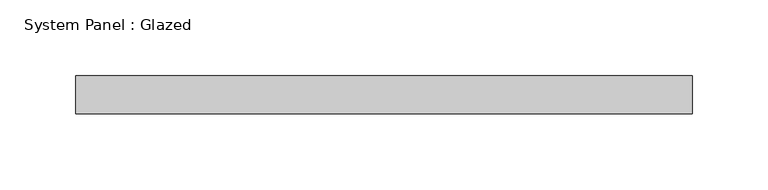
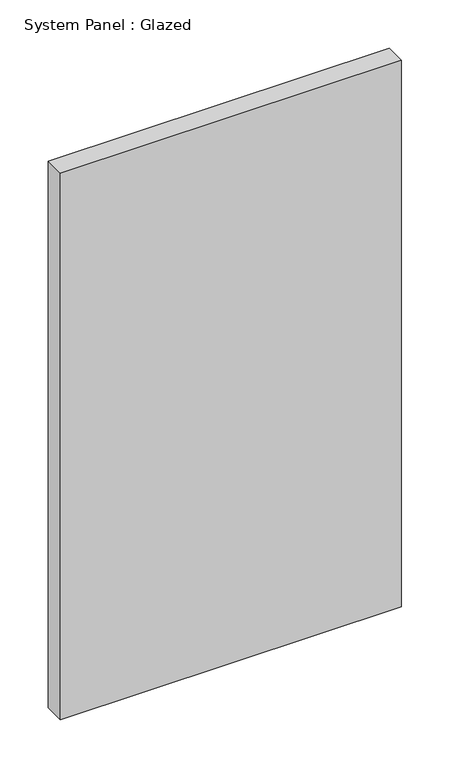
"""IFC4 building model written with IfcOpenShell, lengths in millimetres: plate geometry, System Panel : Glazed."""

from ifc_helpers import new_model, si_unit, origin, origin_with_axes, place, context, project, spatial, polyline, outline, extrude, source, transform, mapped, element, save


def system_panel_glazed_a609a774(model_context):
    return source(origin(), model_context, "Body", "SweptSolid", [
        extrude(outline(polyline([(204.2583333, 19.05), (-204.2583333, 19.05), (-204.2583333, 44.45), (204.2583333, 44.45), (204.2583333, 19.05)])), origin_with_axes(), (0.0, 0.0, 1.0), 692.15),
    ])


if __name__ == "__main__":
    model = new_model("IFC4")
    model_context = context("Model", 3, world=origin())
    ifc_project = project(units=[si_unit("LENGTHUNIT", "METRE", prefix="MILLI")], contexts=[model_context])
    site = spatial("IfcSite", under=ifc_project)
    building = spatial("IfcBuilding", under=site)
    placement = place(None, origin())
    system_panel_glazed_shape = system_panel_glazed_a609a774(model_context)
    element("IfcPlate", 1, ObjectType="System Panel : Glazed", at=placement, inside=building, context=model_context, shape_type="MappedRepresentation", body=[
        mapped(system_panel_glazed_shape, transform((0.0, 0.0, 0.0), x_axis=(1.0, 0.0, 0.0), y_axis=(0.0, 1.0, 0.0), z_axis=(0.0, 0.0, 1.0))),
    ])
    save(model, "model.ifc")

# Revit data of these elements
# Type "System Panel : Glazed"
#   Construction Type Id = "GSP4R"
#   Analytic Construction = "1/8 in Pilkington single glazing"
#   Visual Light Transmittance = 0.9
#   Solar Heat Gain Coefficient = 0.86
#   Heat Transfer Coefficient (U) = 1.18115 BTU/(h·ft²·°F)
#   Define Thermal Properties by = 1
# Element 1 (IfcPlate, "System Panel : Glazed")
#   Materials on its faces: "Glass"
# Materials
#   "Glass": class "Glass", colour RGB 0 128 192, transparency 0.75, Description = "Soda Lime Glass", Cost = 0
